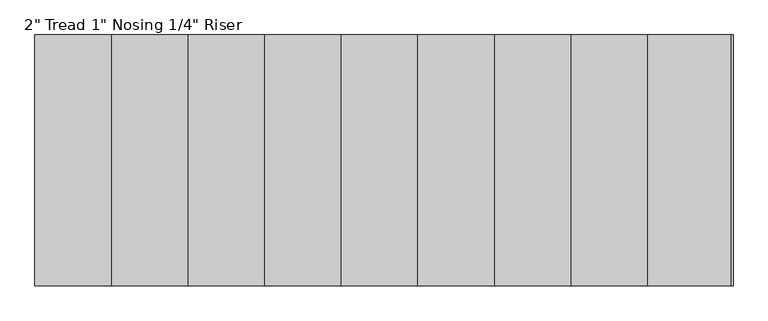
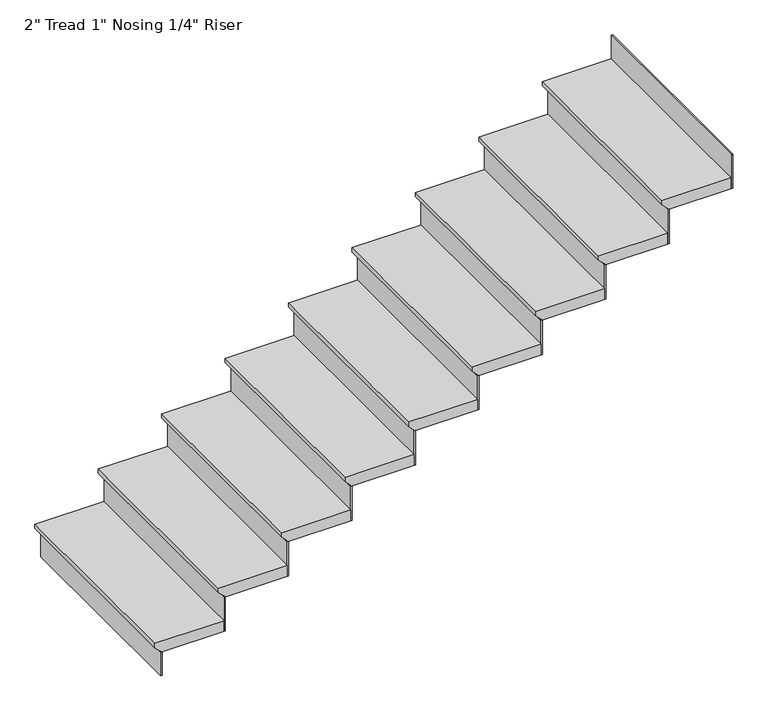
"""IFC4 building model written with IfcOpenShell, lengths in millimetres: stair flight geometry."""

from ifc_helpers import new_model, si_unit, origin, place, context, project, spatial, faceted_brep, source, transform, mapped, element, save


def stair_flight_6ff81285(model_context):
    return source(origin(), model_context, "Body", "Brep", [
        faceted_brep([(-1591.1154463, -4737.3544725, 16142.97), (-1591.1154463, -4737.3544725, 16162.02), (-1591.1154463, -3822.9544725, 16162.02), (-1591.1154463, -3822.9544725, 16142.97), (-1565.7154463, -4737.3544725, 16117.57), (-1565.7154463, -3822.9544725, 16117.57), (-1286.3154463, -4737.3544725, 16162.02), (-1286.3154463, -3822.9544725, 16162.02), (-1565.7154463, -3822.9544725, 16111.22), (-1286.3154463, -3822.9544725, 16111.22), (-1286.3154463, -4737.3544725, 16111.22), (-1565.7154463, -4737.3544725, 16111.22)], [[[0, 1, 2, 3]], [[4, 0, 3, 5]], [[2, 1, 6, 7]], [[8, 9, 10, 11]], [[2, 7, 9, 8, 5, 3]], [[8, 11, 4, 5]], [[6, 1, 0, 4, 11, 10]], [[7, 6, 10, 9]]]),
        faceted_brep([(-1565.7154463, -4737.3544725, 16111.22), (-1565.7154463, -4737.3544725, 16002.0), (-1559.3654463, -4737.3544725, 16002.0), (-1559.3654463, -4737.3544725, 16111.22), (-1565.7154463, -3822.9544725, 16111.22), (-1559.3654463, -3822.9544725, 16111.22), (-1559.3654463, -3822.9544725, 16002.0), (-1565.7154463, -3822.9544725, 16002.0)], [[[0, 1, 2, 3]], [[4, 5, 6, 7]], [[1, 0, 4, 7]], [[2, 1, 7, 6]], [[3, 2, 6, 5]], [[0, 3, 5, 4]]]),
        faceted_brep([(-1286.3154463, -4737.3544725, 16271.24), (-1286.3154463, -4737.3544725, 16111.22), (-1279.9654463, -4737.3544725, 16111.22), (-1279.9654463, -4737.3544725, 16271.24), (-1286.3154463, -3822.9544725, 16271.24), (-1279.9654463, -3822.9544725, 16271.24), (-1279.9654463, -3822.9544725, 16111.22), (-1286.3154463, -3822.9544725, 16111.22)], [[[0, 1, 2, 3]], [[4, 5, 6, 7]], [[1, 0, 4, 7]], [[2, 1, 7, 6]], [[3, 2, 6, 5]], [[0, 3, 5, 4]]]),
        faceted_brep([(-1311.7154463, -3822.9544725, 16322.04), (-1311.7154463, -4737.3544725, 16322.04), (-1006.9154463, -4737.3544725, 16322.04), (-1006.9154463, -3822.9544725, 16322.04), (-1286.3154463, -3822.9544725, 16271.24), (-1006.9154463, -3822.9544725, 16271.24), (-1006.9154463, -4737.3544725, 16271.24), (-1286.3154463, -4737.3544725, 16271.24), (-1286.3154463, -3822.9544725, 16277.59), (-1311.7154463, -3822.9544725, 16302.99), (-1286.3154463, -4737.3544725, 16277.59), (-1311.7154463, -4737.3544725, 16302.99)], [[[0, 1, 2, 3]], [[4, 5, 6, 7]], [[0, 3, 5, 4, 8, 9]], [[4, 7, 10, 8]], [[2, 1, 11, 10, 7, 6]], [[3, 2, 6, 5]], [[11, 1, 0, 9]], [[10, 11, 9, 8]]]),
        faceted_brep([(-1006.9154463, -4737.3544725, 16431.26), (-1006.9154463, -4737.3544725, 16271.24), (-1000.5654463, -4737.3544725, 16271.24), (-1000.5654463, -4737.3544725, 16431.26), (-1006.9154463, -3822.9544725, 16431.26), (-1000.5654463, -3822.9544725, 16431.26), (-1000.5654463, -3822.9544725, 16271.24), (-1006.9154463, -3822.9544725, 16271.24)], [[[0, 1, 2, 3]], [[4, 5, 6, 7]], [[1, 0, 4, 7]], [[2, 1, 7, 6]], [[3, 2, 6, 5]], [[0, 3, 5, 4]]]),
        faceted_brep([(-1032.3154463, -3822.9544725, 16482.06), (-1032.3154463, -4737.3544725, 16482.06), (-727.5154463, -4737.3544725, 16482.06), (-727.5154463, -3822.9544725, 16482.06), (-1006.9154463, -3822.9544725, 16431.26), (-727.5154463, -3822.9544725, 16431.26), (-727.5154463, -4737.3544725, 16431.26), (-1006.9154463, -4737.3544725, 16431.26), (-1006.9154463, -3822.9544725, 16437.61), (-1032.3154463, -3822.9544725, 16463.01), (-1006.9154463, -4737.3544725, 16437.61), (-1032.3154463, -4737.3544725, 16463.01)], [[[0, 1, 2, 3]], [[4, 5, 6, 7]], [[0, 3, 5, 4, 8, 9]], [[4, 7, 10, 8]], [[2, 1, 11, 10, 7, 6]], [[3, 2, 6, 5]], [[11, 1, 0, 9]], [[10, 11, 9, 8]]]),
        faceted_brep([(-727.5154463, -4737.3544725, 16591.28), (-727.5154463, -4737.3544725, 16431.26), (-721.1654463, -4737.3544725, 16431.26), (-721.1654463, -4737.3544725, 16591.28), (-727.5154463, -3822.9544725, 16591.28), (-721.1654463, -3822.9544725, 16591.28), (-721.1654463, -3822.9544725, 16431.26), (-727.5154463, -3822.9544725, 16431.26)], [[[0, 1, 2, 3]], [[4, 5, 6, 7]], [[1, 0, 4, 7]], [[2, 1, 7, 6]], [[3, 2, 6, 5]], [[0, 3, 5, 4]]]),
        faceted_brep([(-752.9154463, -3822.9544725, 16642.08), (-752.9154463, -4737.3544725, 16642.08), (-448.1154463, -4737.3544725, 16642.08), (-448.1154463, -3822.9544725, 16642.08), (-727.5154463, -3822.9544725, 16591.28), (-448.1154463, -3822.9544725, 16591.28), (-448.1154463, -4737.3544725, 16591.28), (-727.5154463, -4737.3544725, 16591.28), (-727.5154463, -3822.9544725, 16597.63), (-752.9154463, -3822.9544725, 16623.03), (-727.5154463, -4737.3544725, 16597.63), (-752.9154463, -4737.3544725, 16623.03)], [[[0, 1, 2, 3]], [[4, 5, 6, 7]], [[0, 3, 5, 4, 8, 9]], [[4, 7, 10, 8]], [[2, 1, 11, 10, 7, 6]], [[3, 2, 6, 5]], [[11, 1, 0, 9]], [[10, 11, 9, 8]]]),
        faceted_brep([(-448.1154463, -4737.3544725, 16751.3), (-448.1154463, -4737.3544725, 16591.28), (-441.7654463, -4737.3544725, 16591.28), (-441.7654463, -4737.3544725, 16751.3), (-448.1154463, -3822.9544725, 16751.3), (-441.7654463, -3822.9544725, 16751.3), (-441.7654463, -3822.9544725, 16591.28), (-448.1154463, -3822.9544725, 16591.28)], [[[0, 1, 2, 3]], [[4, 5, 6, 7]], [[1, 0, 4, 7]], [[2, 1, 7, 6]], [[3, 2, 6, 5]], [[0, 3, 5, 4]]]),
        faceted_brep([(-473.5154463, -3822.9544725, 16802.1), (-473.5154463, -4737.3544725, 16802.1), (-168.7154463, -4737.3544725, 16802.1), (-168.7154463, -3822.9544725, 16802.1), (-448.1154463, -3822.9544725, 16751.3), (-168.7154463, -3822.9544725, 16751.3), (-168.7154463, -4737.3544725, 16751.3), (-448.1154463, -4737.3544725, 16751.3), (-448.1154463, -3822.9544725, 16757.65), (-473.5154463, -3822.9544725, 16783.05), (-448.1154463, -4737.3544725, 16757.65), (-473.5154463, -4737.3544725, 16783.05)], [[[0, 1, 2, 3]], [[4, 5, 6, 7]], [[0, 3, 5, 4, 8, 9]], [[4, 7, 10, 8]], [[2, 1, 11, 10, 7, 6]], [[3, 2, 6, 5]], [[11, 1, 0, 9]], [[10, 11, 9, 8]]]),
        faceted_brep([(-168.7154463, -4737.3544725, 16911.32), (-168.7154463, -4737.3544725, 16751.3), (-162.3654463, -4737.3544725, 16751.3), (-162.3654463, -4737.3544725, 16911.32), (-168.7154463, -3822.9544725, 16911.32), (-162.3654463, -3822.9544725, 16911.32), (-162.3654463, -3822.9544725, 16751.3), (-168.7154463, -3822.9544725, 16751.3)], [[[0, 1, 2, 3]], [[4, 5, 6, 7]], [[1, 0, 4, 7]], [[2, 1, 7, 6]], [[3, 2, 6, 5]], [[0, 3, 5, 4]]]),
        faceted_brep([(-194.1154463, -3822.9544725, 16962.12), (-194.1154463, -4737.3544725, 16962.12), (110.6845537, -4737.3544725, 16962.12), (110.6845537, -3822.9544725, 16962.12), (-168.7154463, -3822.9544725, 16911.32), (110.6845537, -3822.9544725, 16911.32), (110.6845537, -4737.3544725, 16911.32), (-168.7154463, -4737.3544725, 16911.32), (-168.7154463, -3822.9544725, 16917.67), (-194.1154463, -3822.9544725, 16943.07), (-168.7154463, -4737.3544725, 16917.67), (-194.1154463, -4737.3544725, 16943.07)], [[[0, 1, 2, 3]], [[4, 5, 6, 7]], [[0, 3, 5, 4, 8, 9]], [[4, 7, 10, 8]], [[2, 1, 11, 10, 7, 6]], [[3, 2, 6, 5]], [[11, 1, 0, 9]], [[10, 11, 9, 8]]]),
        faceted_brep([(110.6845537, -4737.3544725, 17071.34), (110.6845537, -4737.3544725, 16911.32), (117.0345537, -4737.3544725, 16911.32), (117.0345537, -4737.3544725, 17071.34), (110.6845537, -3822.9544725, 17071.34), (117.0345537, -3822.9544725, 17071.34), (117.0345537, -3822.9544725, 16911.32), (110.6845537, -3822.9544725, 16911.32)], [[[0, 1, 2, 3]], [[4, 5, 6, 7]], [[1, 0, 4, 7]], [[2, 1, 7, 6]], [[3, 2, 6, 5]], [[0, 3, 5, 4]]]),
        faceted_brep([(85.2845537, -3822.9544725, 17122.14), (85.2845537, -4737.3544725, 17122.14), (390.0845537, -4737.3544725, 17122.14), (390.0845537, -3822.9544725, 17122.14), (110.6845537, -3822.9544725, 17071.34), (390.0845537, -3822.9544725, 17071.34), (390.0845537, -4737.3544725, 17071.34), (110.6845537, -4737.3544725, 17071.34), (110.6845537, -3822.9544725, 17077.69), (85.2845537, -3822.9544725, 17103.09), (110.6845537, -4737.3544725, 17077.69), (85.2845537, -4737.3544725, 17103.09)], [[[0, 1, 2, 3]], [[4, 5, 6, 7]], [[0, 3, 5, 4, 8, 9]], [[4, 7, 10, 8]], [[2, 1, 11, 10, 7, 6]], [[3, 2, 6, 5]], [[11, 1, 0, 9]], [[10, 11, 9, 8]]]),
        faceted_brep([(390.0845537, -4737.3544725, 17231.36), (390.0845537, -4737.3544725, 17071.34), (396.4345537, -4737.3544725, 17071.34), (396.4345537, -4737.3544725, 17231.36), (390.0845537, -3822.9544725, 17231.36), (396.4345537, -3822.9544725, 17231.36), (396.4345537, -3822.9544725, 17071.34), (390.0845537, -3822.9544725, 17071.34)], [[[0, 1, 2, 3]], [[4, 5, 6, 7]], [[1, 0, 4, 7]], [[2, 1, 7, 6]], [[3, 2, 6, 5]], [[0, 3, 5, 4]]]),
        faceted_brep([(364.6845537, -3822.9544725, 17282.16), (364.6845537, -4737.3544725, 17282.16), (669.4845537, -4737.3544725, 17282.16), (669.4845537, -3822.9544725, 17282.16), (390.0845537, -3822.9544725, 17231.36), (669.4845537, -3822.9544725, 17231.36), (669.4845537, -4737.3544725, 17231.36), (390.0845537, -4737.3544725, 17231.36), (390.0845537, -3822.9544725, 17237.71), (364.6845537, -3822.9544725, 17263.11), (390.0845537, -4737.3544725, 17237.71), (364.6845537, -4737.3544725, 17263.11)], [[[0, 1, 2, 3]], [[4, 5, 6, 7]], [[0, 3, 5, 4, 8, 9]], [[4, 7, 10, 8]], [[2, 1, 11, 10, 7, 6]], [[3, 2, 6, 5]], [[11, 1, 0, 9]], [[10, 11, 9, 8]]]),
        faceted_brep([(948.8845537, -4737.3544725, 17551.4), (948.8845537, -4737.3544725, 17391.38), (955.2345537, -4737.3544725, 17391.38), (955.2345537, -4737.3544725, 17551.4), (948.8845537, -3822.9544725, 17551.4), (955.2345537, -3822.9544725, 17551.4), (955.2345537, -3822.9544725, 17391.38), (948.8845537, -3822.9544725, 17391.38)], [[[0, 1, 2, 3]], [[4, 5, 6, 7]], [[1, 0, 4, 7]], [[2, 1, 7, 6]], [[3, 2, 6, 5]], [[0, 3, 5, 4]]]),
        faceted_brep([(669.4845537, -4737.3544725, 17391.38), (669.4845537, -4737.3544725, 17231.36), (675.8345537, -4737.3544725, 17231.36), (675.8345537, -4737.3544725, 17391.38), (669.4845537, -3822.9544725, 17391.38), (675.8345537, -3822.9544725, 17391.38), (675.8345537, -3822.9544725, 17231.36), (669.4845537, -3822.9544725, 17231.36)], [[[0, 1, 2, 3]], [[4, 5, 6, 7]], [[1, 0, 4, 7]], [[2, 1, 7, 6]], [[3, 2, 6, 5]], [[0, 3, 5, 4]]]),
        faceted_brep([(948.8845537, -3822.9544725, 17442.18), (923.4845537, -3822.9544725, 17442.18), (644.0845537, -3822.9544725, 17442.18), (644.0845537, -4737.3544725, 17442.18), (948.8845537, -4737.3544725, 17442.18), (923.4845537, -3822.9544725, 17391.38), (948.8845537, -3822.9544725, 17391.38), (948.8845537, -4737.3544725, 17391.38), (669.4845537, -4737.3544725, 17391.38), (669.4845537, -3822.9544725, 17391.38), (669.4845537, -3822.9544725, 17397.73), (644.0845537, -3822.9544725, 17423.13), (669.4845537, -4737.3544725, 17397.73), (644.0845537, -4737.3544725, 17423.13)], [[[0, 1, 2, 3, 4]], [[5, 6, 7, 8, 9]], [[1, 0, 6, 5]], [[2, 1, 5, 9, 10, 11]], [[9, 8, 12, 10]], [[4, 3, 13, 12, 8, 7]], [[0, 4, 7, 6]], [[13, 3, 2, 11]], [[12, 13, 11, 10]]]),
    ])


if __name__ == "__main__":
    model = new_model("IFC4")
    model_context = context("Model", 3, world=origin())
    ifc_project = project(units=[si_unit("LENGTHUNIT", "METRE", prefix="MILLI")], contexts=[model_context])
    site = spatial("IfcSite", under=ifc_project)
    building = spatial("IfcBuilding", under=site)
    placement = place(None, origin())
    stair_flight_shape = stair_flight_6ff81285(model_context)
    element("IfcStairFlight", 1, ObjectType="2\" Tread 1\" Nosing 1/4\" Riser", at=placement, inside=building, context=model_context, shape_type="MappedRepresentation", body=[
        mapped(stair_flight_shape, transform((0.0, 0.0, 0.0), x_axis=(1.0, 0.0, 0.0), y_axis=(0.0, 1.0, 0.0), z_axis=(0.0, 0.0, 1.0))),
    ])
    save(model, "model.ifc")
